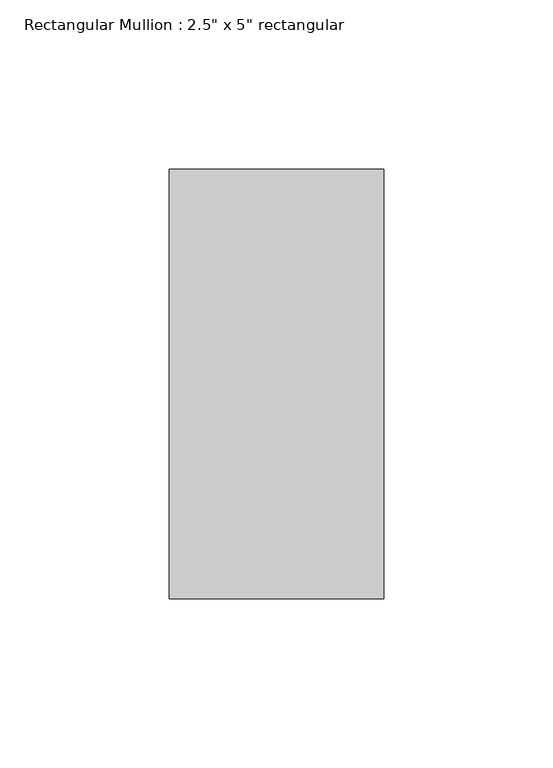
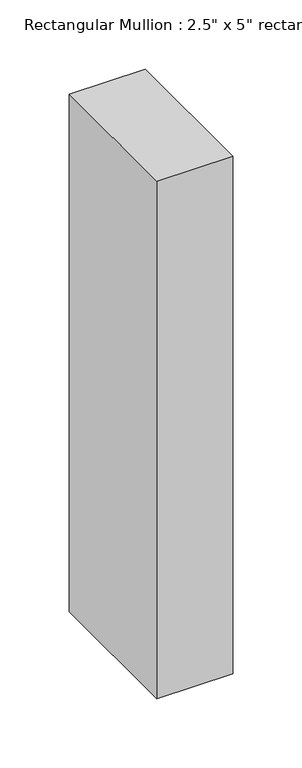
"""IFC4 building model written with IfcOpenShell, lengths in millimetres: member geometry."""

from ifc_helpers import new_model, si_unit, frame, origin, place, context, project, spatial, polyline, outline, extrude, source, transform, mapped, element, save


def member_ffd4c858(model_context):
    return source(origin(), model_context, "Body", "SweptSolid", [
        extrude(outline(polyline([(31.75, 63.5), (31.75, -63.5), (-31.75, -63.5), (-31.75, 63.5), (31.75, 63.5)])), frame((0.0, 0.0, -457.2), z_axis=(0.0, 0.0, 1.0), x_axis=(1.0, 0.0, 0.0)), (0.0, 0.0, 1.0), 457.2),
    ])


if __name__ == "__main__":
    model = new_model("IFC4")
    model_context = context("Model", 3, world=origin())
    ifc_project = project(units=[si_unit("LENGTHUNIT", "METRE", prefix="MILLI")], contexts=[model_context])
    site = spatial("IfcSite", under=ifc_project)
    building = spatial("IfcBuilding", under=site)
    placement = place(None, origin())
    member_shape = member_ffd4c858(model_context)
    element("IfcMember", 1, ObjectType="Rectangular Mullion : 2.5\" x 5\" rectangular", at=placement, inside=building, context=model_context, shape_type="MappedRepresentation", body=[
        mapped(member_shape, transform((0.0, 0.0, 0.0), x_axis=(1.0, 0.0, 0.0), y_axis=(0.0, 1.0, 0.0), z_axis=(0.0, 0.0, 1.0))),
    ])
    save(model, "model.ifc")

# Revit data of these elements
# Type "Rectangular Mullion : 2.5\" x 5\" rectangular"
#   built-in parameter 1007304 = 0.416667 (stored number, unit not read)
#   built-in parameter 1007301 = 0.104167 (stored number, unit not read)
#   built-in parameter 1007300 = 0.104167 (stored number, unit not read)
